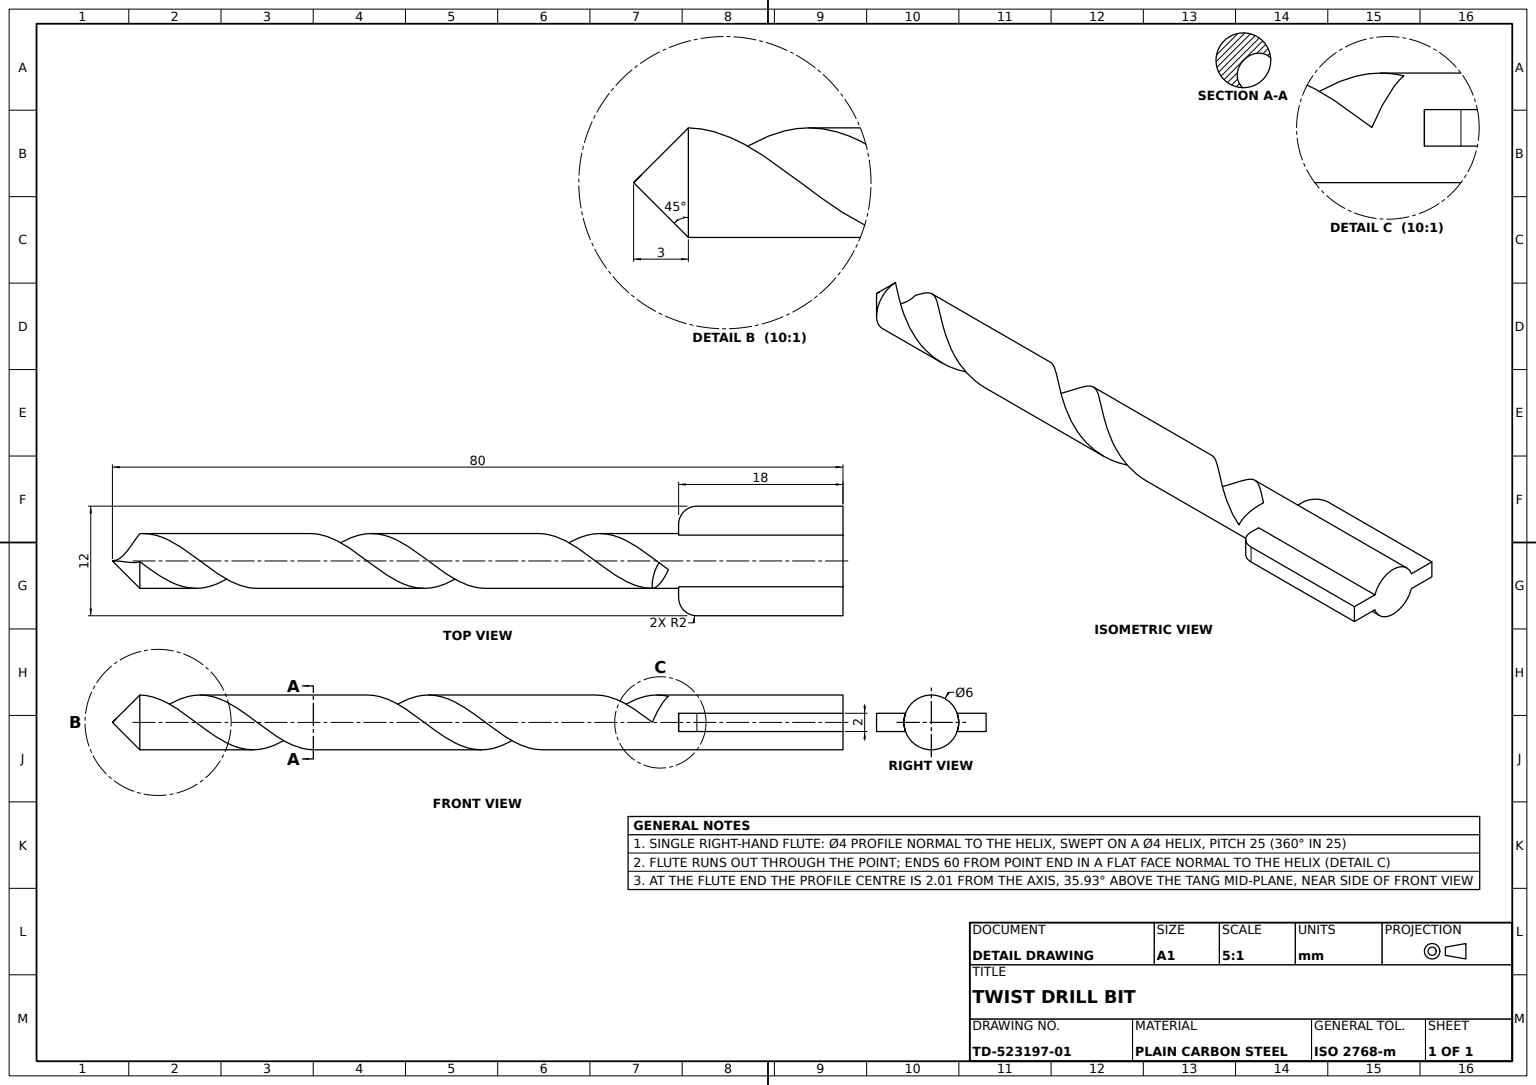
SolidWorks part; units mm, degrees
material "Plain Carbon Steel"
ref_plane "Front Plane" through (0, 0, 0) normal (0, 0, 1) x (1, 0, 0)
ref_plane "Top Plane" through (0, 0, 0) normal (0, 1, 0) x (1, 0, 0)
ref_plane "Right Plane" through (0, 0, 0) normal (1, 0, 0) x (0, 0, -1)
sketch "Body Profile Ø6" plane through (0, 0, 0) normal (0, 1, 0) x (1, 0, 0)
  circle A0 centre (0, 0) radius 3
  dimension "D1" = 6
extrude "Drill Body Ø6 x 80" add sketch "Body Profile Ø6" along normal blind 80
sketch "Reference Helix Circle" plane through (0, 80, 0) normal (0, 1, 0) x (1, 0, 0)
  circle A0 centre (0, 0) radius 3 construction
  circle A1 centre (0, 0) radius 3
curve "Reference Helix Pitch 25" pitch 25 height 60 turns 2.4
ref_plane "Plane1" through (0, 80, 3) normal (-0.602, -0.7985, 0) x (-0.7985, 0.602, 0)
ref_plane "Plane2" through (38.4565, 51.0045, 0) normal (-0.602, -0.7985, 0) x (-0.7985, 0.602, 0)
sketch "Flute Helix Circle Ø4" plane through (0, 80, 0) normal (0, 1, 0) x (1, 0, 0)
  circle A0 centre (0, 0) radius 2
  dimension "D1" = 4
chamfer "Tip Chamfer 3x45°" distance 3 angle 45 1 edges at (0, 80, 3)
curve "Flute Helix Pitch 25" pitch 25 height 60 turns 2.4
ref_plane "Plane4" through (0, 80, 2) normal (-0.4491, -0.8935, 0) x (-0.8935, 0.4491, 0)
ref_plane "Plane5" through (0, 80, 2) normal (-0.4491, -0.8935, 0) x (-0.8935, 0.4491, 0)
sketch "Flute Profile Ø4" plane through (0, 80, 2) normal (-0.4491, -0.8935, 0) x (-0.8935, 0.4491, 0)
  circle A0 centre (-0.0003, -0.0101) radius 2
  dimension "D1" = 4
  dimension "D2" = 35.9285
  dimension "D3" = 2.0101
sweep "Helical Flute" cut profiles "Flute Profile Ø4" path "Flute Helix Pitch 25"
sketch "Tang Profile 12x18" plane through (0, 0, 0) normal (1, 0, 0) x (0, 0, -1)
  line L1 (-6, 18) -> (6, 18)
  line L2 (-6, 18) -> (-6, 0)
  line L3 (-6, 0) -> (6, 0)
  line L4 (6, 18) -> (6, 0)
  point P4 (0, 0)
  dimension "D1" = 12
  dimension "D2" = 18
extrude "Drive Tang 2mm" add sketch "Tang Profile 12x18" along normal mid plane 2
fillet "Tang Fillet R2 A" radius 2 1 edges at (0, 18, 6)
fillet "Tang Fillet R2 B" radius 2 1 edges at (0, 18, -6)
